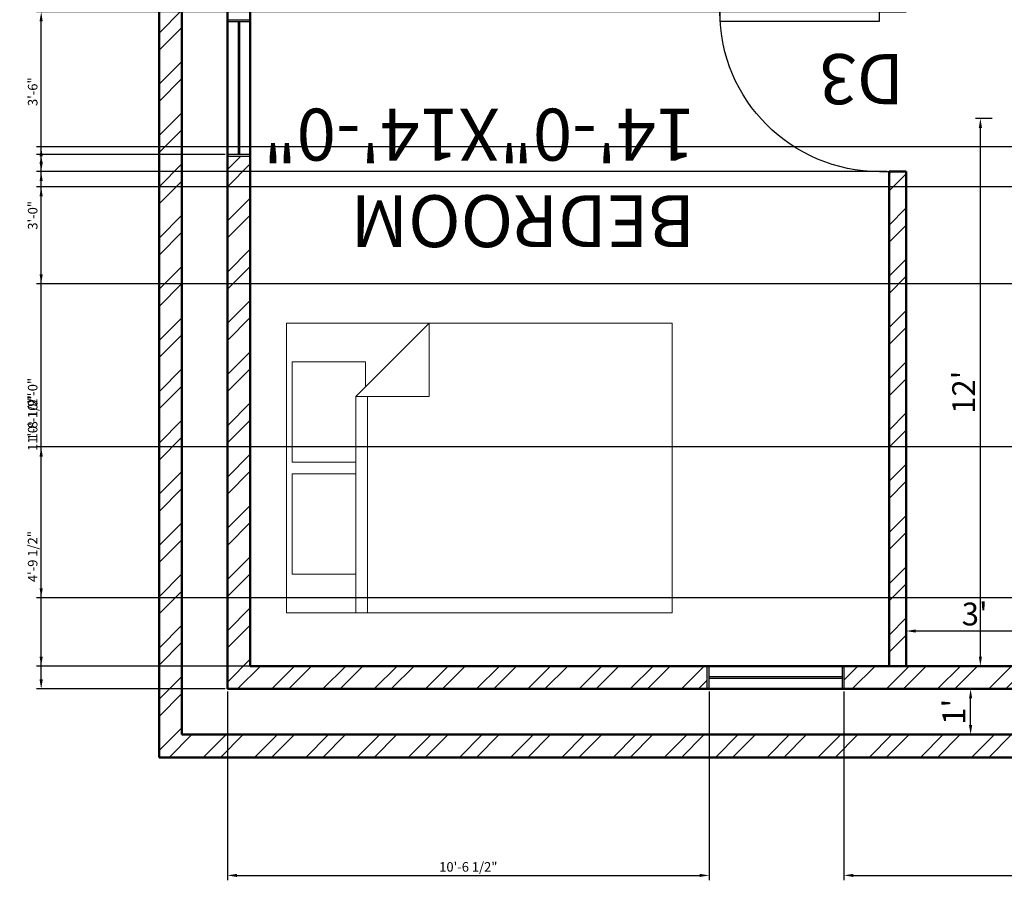
# Model space of a CAD drawing. Units: inches. Extents: x 244 to 2800, y 1060 to 1700.
# Tile 6 of 13: x 1476 to 1735, y 1060 to 1287. Entities that reach past the tile are written whole.
import ezdxf

# ---------------------------------------------------------------- set-up
doc = ezdxf.new("R2010")
doc.units = ezdxf.units.IN
for name, color, linetype, lineweight in [('A-ANNO-DIMS', 2, 'Continuous', 18), ('A-ANNO-TEXT', 1, 'Continuous', 18), ('A-DOOR', 5, 'Continuous', 25), ('A-FURN', 9, 'Continuous', 18), ('A-GLAZ', 3, 'Continuous', 25), ('A-WALL', 7, 'Continuous', 50), ('A-WALL-PATT', 8, 'Continuous', 13)]:
    doc.layers.add(name, color=color, linetype=linetype, lineweight=lineweight)
doc.styles.get("Standard").update_dxf_attribs({"font": 'arial.ttf'})
doc.dimstyles.new('ISO-25', dxfattribs={"dimtxt": 2.5, "dimasz": 2.5, "dimexe": 1.25, "dimexo": 0.625, "dimtad": 1, "dimlunit": 4, "dimtxsty": 'Standard', "dimcen": 2.5, "dimadec": 0, "dimazin": 0, "dimtfac": 1, "dimtmove": 0, "dimatfit": 3, "dimfxl": 1, "dimarcsym": 0})

# ---------------------------------------------------------------- blocks, each defined once
blk = doc.blocks.new('*U2')
for p, q in [((0, 0), (0, -5)), ((30, 0), (30, -5))]:
    blk.add_line(p, q)
blk.add_lwpolyline([(0, 0), (0, 30), (1.75, 30), (1.75, 0)], close=True)
blk.add_arc((0, 0), 30, 0, 90)
blk = doc.blocks.new('Bed - Queen')
for p, q in [((0, -80.00003), (0, 0)), ((0, 0), (59.99999, 0)), ((59.99999, 0), (59.99999, -80.00003)), ((7.99999, -1.2), (28.79998, -1.2)), ((7.99999, -14.4), (7.99999, -1.2)), ((28.79998, -1.2), (28.79998, -14.4)), ((31.19999, -1.2), (51.99999, -1.2)), ((31.19999, -14.4), (31.19999, -1.2)), ((51.99999, -1.2), (51.99999, -16.4)), ((0, -14.4), (44.8, -14.4)), ((59.99999, -29.6), (44.8, -14.4)), ((44.8, -14.4), (44.8, -29.6)), ((44.8, -16.8), (0, -16.8)), ((51.99999, -16.4), (46.79936, -16.4)), ((44.8, -29.6), (59.99999, -29.6)), ((59.99999, -80.00003), (0, -80.00003))]:
    blk.add_line(p, q)
blk = doc.blocks.new('*D37')
at = {"layer": 'A-ANNO-DIMS', "color": 0, "lineweight": -2, "transparency": 16777216}
for p, q in [((1731.11, 1110.99), (1724.58, 1110.99)), ((1725.83, 1101.49), (1725.83, 1108.49)), ((1731.11, 1098.99), (1724.58, 1098.99))]:
    blk.add_line(p, q, dxfattribs=at)
at = {"layer": 'A-ANNO-DIMS', "color": 0, "transparency": 16777216}
for points in [[(1725.42, 1108.49), (1726.25, 1108.49), (1725.83, 1110.99)], [(1725.42, 1101.49), (1726.25, 1101.49), (1725.83, 1098.99)]]:
    blk.add_solid(points, dxfattribs=at)
at = {"layer": 'Defpoints', "color": 0, "transparency": 16777216}
for p in [(1725.83, 1110.99), (1731.74, 1110.99), (1731.74, 1098.99)]:
    blk.add_point(p, dxfattribs=at)
at = {"layer": 'A-ANNO-DIMS', "color": 0, "transparency": 16777216, "insert": (1722.2, 1104.99), "char_height": 6, "attachment_point": 5, "rotation": 90}
blk.add_mtext("1'", dxfattribs=at)
blk = doc.blocks.new('*D38')
at = {"layer": 'A-ANNO-DIMS', "color": 0, "lineweight": -2, "transparency": 16777216}
for p, q in [((1708.9, 1124.22), (1708.9, 1127.48)), ((1744.9, 1124.22), (1744.9, 1127.48)), ((1742.4, 1126.23), (1711.4, 1126.23))]:
    blk.add_line(p, q, dxfattribs=at)
at = {"layer": 'A-ANNO-DIMS', "color": 0, "transparency": 16777216}
for points in [[(1711.4, 1126.65), (1711.4, 1125.81), (1708.9, 1126.23)], [(1742.4, 1126.65), (1742.4, 1125.81), (1744.9, 1126.23)]]:
    blk.add_solid(points, dxfattribs=at)
at = {"layer": 'Defpoints', "color": 0, "transparency": 16777216}
for p in [(1708.9, 1126.23), (1708.9, 1123.59), (1744.9, 1123.59)]:
    blk.add_point(p, dxfattribs=at)
at = {"layer": 'A-ANNO-DIMS', "color": 0, "transparency": 16777216, "insert": (1726.9, 1129.92), "char_height": 6, "attachment_point": 5}
blk.add_mtext("3'", dxfattribs=at)
blk = doc.blocks.new('*D39')
at = {"layer": 'A-ANNO-DIMS', "color": 0, "lineweight": -2, "transparency": 16777216}
for p, q in [((1731.52, 1260.99), (1727.15, 1260.99)), ((1728.4, 1119.49), (1728.4, 1258.49)), ((1731.92, 1116.99), (1727.15, 1116.99))]:
    blk.add_line(p, q, dxfattribs=at)
at = {"layer": 'A-ANNO-DIMS', "color": 0, "transparency": 16777216}
for points in [[(1727.99, 1258.49), (1728.82, 1258.49), (1728.4, 1260.99)], [(1727.99, 1119.49), (1728.82, 1119.49), (1728.4, 1116.99)]]:
    blk.add_solid(points, dxfattribs=at)
at = {"layer": 'Defpoints', "color": 0, "transparency": 16777216}
for p in [(1728.4, 1260.99), (1732.15, 1260.99), (1732.55, 1116.99)]:
    blk.add_point(p, dxfattribs=at)
at = {"layer": 'A-ANNO-DIMS', "color": 0, "transparency": 16777216, "insert": (1724.77, 1188.99), "char_height": 6, "attachment_point": 5, "rotation": 90}
blk.add_mtext("12'", dxfattribs=at)
blk = doc.blocks.new('WIN-36')
for p, q in [((0, 0), (0, 6)), ((0, 6), (35.94, 6)), ((35.94, 6), (35.94, 0)), ((35.94, 0), (0, 0))]:
    blk.add_line(p, q)
blk = doc.blocks.new('*D81')
at = {"layer": 'A-ANNO-DIMS', "color": 0, "lineweight": -2, "transparency": 16777216}
for p, q in [((1529.77, 1251.47), (1480.15, 1251.47)), ((1481.4, 1113.49), (1481.4, 1248.97)), ((1529.77, 1110.99), (1480.15, 1110.99))]:
    blk.add_line(p, q, dxfattribs=at)
at = {"layer": 'A-ANNO-DIMS', "color": 0, "transparency": 16777216}
for points in [[(1480.98, 1248.97), (1481.81, 1248.97), (1481.4, 1251.47)], [(1480.98, 1113.49), (1481.81, 1113.49), (1481.4, 1110.99)]]:
    blk.add_solid(points, dxfattribs=at)
at = {"layer": 'Defpoints', "color": 0, "transparency": 16777216}
for p in [(1481.4, 1251.47), (1530.4, 1251.47), (1530.4, 1110.99)]:
    blk.add_point(p, dxfattribs=at)
at = {"layer": 'A-ANNO-DIMS', "color": 0, "transparency": 16777216, "insert": (1479.48, 1181.23), "char_height": 2.5, "attachment_point": 5, "rotation": 90}
blk.add_mtext('11\'-8 1/2"', dxfattribs=at)
blk = doc.blocks.new('*D85')
at = {"layer": 'A-ANNO-DIMS', "color": 0, "lineweight": -2, "transparency": 16777216}
for p, q in [((1537.02, 1291.99), (2024.65, 1291.99)), ((2023.4, 1119.49), (2023.4, 1289.49)), ((1537.02, 1116.99), (2024.65, 1116.99))]:
    blk.add_line(p, q, dxfattribs=at)
at = {"layer": 'A-ANNO-DIMS', "color": 0, "transparency": 16777216}
for points in [[(2022.98, 1289.49), (2023.81, 1289.49), (2023.4, 1291.99)], [(2022.98, 1119.49), (2023.81, 1119.49), (2023.4, 1116.99)]]:
    blk.add_solid(points, dxfattribs=at)
at = {"layer": 'Defpoints', "color": 0, "transparency": 16777216}
for p in [(1536.4, 1291.99), (2023.4, 1291.99), (1536.4, 1116.99)]:
    blk.add_point(p, dxfattribs=at)
at = {"layer": 'A-ANNO-DIMS', "color": 0, "transparency": 16777216, "insert": (2021.52, 1204.49), "char_height": 2.5, "attachment_point": 5, "rotation": 90}
blk.add_mtext('14\'-7"', dxfattribs=at)
blk = doc.blocks.new('*D91')
at = {"layer": 'A-ANNO-DIMS', "color": 0, "lineweight": -2, "transparency": 16777216}
for p, q in [((1703.77, 1246.99), (1480.15, 1246.99)), ((1481.4, 1119.49), (1481.4, 1244.49)), ((1703.77, 1116.99), (1480.15, 1116.99))]:
    blk.add_line(p, q, dxfattribs=at)
at = {"layer": 'A-ANNO-DIMS', "color": 0, "transparency": 16777216}
for points in [[(1480.98, 1244.49), (1481.81, 1244.49), (1481.4, 1246.99)], [(1480.98, 1119.49), (1481.81, 1119.49), (1481.4, 1116.99)]]:
    blk.add_solid(points, dxfattribs=at)
at = {"layer": 'Defpoints', "color": 0, "transparency": 16777216}
for p in [(1481.4, 1246.99), (1704.4, 1246.99), (1704.4, 1116.99)]:
    blk.add_point(p, dxfattribs=at)
at = {"layer": 'A-ANNO-DIMS', "color": 0, "transparency": 16777216, "insert": (1479.49, 1181.99), "char_height": 2.5, "attachment_point": 5, "rotation": 90}
blk.add_mtext('10\'-10"', dxfattribs=at)
blk = doc.blocks.new('*D92')
at = {"layer": 'A-ANNO-DIMS', "color": 0, "lineweight": -2, "transparency": 16777216}
for p, q in [((1703.77, 1288.99), (1480.15, 1288.99)), ((1481.4, 1249.49), (1481.4, 1286.49)), ((1703.77, 1246.99), (1480.15, 1246.99))]:
    blk.add_line(p, q, dxfattribs=at)
at = {"layer": 'A-ANNO-DIMS', "color": 0, "transparency": 16777216}
for points in [[(1480.98, 1286.49), (1481.81, 1286.49), (1481.4, 1288.99)], [(1480.98, 1249.49), (1481.81, 1249.49), (1481.4, 1246.99)]]:
    blk.add_solid(points, dxfattribs=at)
at = {"layer": 'Defpoints', "color": 0, "transparency": 16777216}
for p in [(1481.4, 1288.99), (1704.4, 1288.99), (1704.4, 1246.99)]:
    blk.add_point(p, dxfattribs=at)
at = {"layer": 'A-ANNO-DIMS', "color": 0, "transparency": 16777216, "insert": (1479.49, 1267.99), "char_height": 2.5, "attachment_point": 5, "rotation": 90}
blk.add_mtext('3\'-6"', dxfattribs=at)
blk = doc.blocks.new('*D94')
at = {"layer": 'A-ANNO-DIMS', "color": 0, "lineweight": -2, "transparency": 16777216}
for p, q in [((1530.4, 1110.36), (1530.4, 1060.74)), ((1657.07, 1110.36), (1657.07, 1060.74)), ((1532.9, 1061.99), (1654.57, 1061.99))]:
    blk.add_line(p, q, dxfattribs=at)
at = {"layer": 'A-ANNO-DIMS', "color": 0, "transparency": 16777216}
for points in [[(1532.9, 1062.4), (1532.9, 1061.57), (1530.4, 1061.99)], [(1654.57, 1062.4), (1654.57, 1061.57), (1657.07, 1061.99)]]:
    blk.add_solid(points, dxfattribs=at)
at = {"layer": 'Defpoints', "color": 0, "transparency": 16777216}
for p in [(1530.4, 1110.99), (1657.07, 1110.99), (1657.07, 1061.99)]:
    blk.add_point(p, dxfattribs=at)
at = {"layer": 'A-ANNO-DIMS', "color": 0, "transparency": 16777216, "insert": (1593.74, 1063.9), "char_height": 2.5, "attachment_point": 5}
blk.add_mtext('10\'-6 1/2"', dxfattribs=at)
blk = doc.blocks.new('*D95')
at = {"layer": 'A-ANNO-DIMS', "color": 0, "lineweight": -2, "transparency": 16777216}
for p, q in [((1692.52, 1110.36), (1692.52, 1060.74)), ((1795.9, 1110.36), (1795.9, 1060.74)), ((1695.02, 1061.99), (1793.4, 1061.99))]:
    blk.add_line(p, q, dxfattribs=at)
at = {"layer": 'A-ANNO-DIMS', "color": 0, "transparency": 16777216}
for points in [[(1695.02, 1062.4), (1695.02, 1061.57), (1692.52, 1061.99)], [(1793.4, 1062.4), (1793.4, 1061.57), (1795.9, 1061.99)]]:
    blk.add_solid(points, dxfattribs=at)
at = {"layer": 'Defpoints', "color": 0, "transparency": 16777216}
for p in [(1692.52, 1110.99), (1795.9, 1110.99), (1795.9, 1061.99)]:
    blk.add_point(p, dxfattribs=at)
at = {"layer": 'A-ANNO-DIMS', "color": 0, "transparency": 16777216, "insert": (1744.21, 1063.9), "char_height": 2.5, "attachment_point": 5}
blk.add_mtext('8\'-7 1/2"', dxfattribs=at)
blk = doc.blocks.new('*D103')
at = {"layer": 'A-ANNO-DIMS', "color": 0, "lineweight": -2, "transparency": 16777216}
for p, q in [((1985.77, 1242.99), (1480.15, 1242.99)), ((1481.4, 1137.49), (1481.4, 1240.49)), ((1985.77, 1134.99), (1480.15, 1134.99))]:
    blk.add_line(p, q, dxfattribs=at)
at = {"layer": 'A-ANNO-DIMS', "color": 0, "transparency": 16777216}
for points in [[(1480.98, 1240.49), (1481.81, 1240.49), (1481.4, 1242.99)], [(1480.98, 1137.49), (1481.81, 1137.49), (1481.4, 1134.99)]]:
    blk.add_solid(points, dxfattribs=at)
at = {"layer": 'Defpoints', "color": 0, "transparency": 16777216}
for p in [(1481.4, 1242.99), (1986.4, 1242.99), (1986.4, 1134.99)]:
    blk.add_point(p, dxfattribs=at)
at = {"layer": 'A-ANNO-DIMS', "color": 0, "transparency": 16777216, "insert": (1479.49, 1188.99), "char_height": 2.5, "attachment_point": 5, "rotation": 90}
blk.add_mtext('9\'-0"', dxfattribs=at)
blk = doc.blocks.new('*D105')
at = {"layer": 'A-ANNO-DIMS', "color": 0, "lineweight": -2, "transparency": 16777216}
for p, q in [((1831.27, 1253.49), (1480.15, 1253.49)), ((1481.4, 1219.99), (1481.4, 1250.99)), ((1831.27, 1217.49), (1480.15, 1217.49))]:
    blk.add_line(p, q, dxfattribs=at)
at = {"layer": 'A-ANNO-DIMS', "color": 0, "transparency": 16777216}
for points in [[(1480.98, 1250.99), (1481.81, 1250.99), (1481.4, 1253.49)], [(1480.98, 1219.99), (1481.81, 1219.99), (1481.4, 1217.49)]]:
    blk.add_solid(points, dxfattribs=at)
at = {"layer": 'Defpoints', "color": 0, "transparency": 16777216}
for p in [(1481.4, 1253.49), (1831.9, 1253.49), (1831.9, 1217.49)]:
    blk.add_point(p, dxfattribs=at)
at = {"layer": 'A-ANNO-DIMS', "color": 0, "transparency": 16777216, "insert": (1479.49, 1235.49), "char_height": 2.5, "attachment_point": 5, "rotation": 90}
blk.add_mtext('3\'-0"', dxfattribs=at)
blk = doc.blocks.new('*D106')
at = {"layer": 'A-ANNO-DIMS', "color": 0, "lineweight": -2, "transparency": 16777216}
for p, q in [((1895.77, 1174.6), (1480.15, 1174.6)), ((1481.4, 1119.49), (1481.4, 1172.1)), ((1895.77, 1116.99), (1480.15, 1116.99))]:
    blk.add_line(p, q, dxfattribs=at)
at = {"layer": 'A-ANNO-DIMS', "color": 0, "transparency": 16777216}
for points in [[(1480.98, 1172.1), (1481.81, 1172.1), (1481.4, 1174.6)], [(1480.98, 1119.49), (1481.81, 1119.49), (1481.4, 1116.99)]]:
    blk.add_solid(points, dxfattribs=at)
at = {"layer": 'Defpoints', "color": 0, "transparency": 16777216}
for p in [(1481.4, 1174.6), (1896.4, 1174.6), (1896.4, 1116.99)]:
    blk.add_point(p, dxfattribs=at)
at = {"layer": 'A-ANNO-DIMS', "color": 0, "transparency": 16777216, "insert": (1479.48, 1145.79), "char_height": 2.5, "attachment_point": 5, "rotation": 90}
blk.add_mtext('4\'-9 1/2"', dxfattribs=at)

msp = doc.modelspace()

# ---------------------------------------------------------------- hatches: boundary and pattern name
at = {"layer": 'A-WALL-PATT'}
h = msp.add_hatch(dxfattribs=at)
h.set_pattern_fill('ANSI32', color=256)
h.paths.add_polyline_path([(1992.396, 1092.986), (1992.396, 1632.986), (1512.396, 1632.986), (1512.396, 1092.986)])
h.paths.add_polyline_path([(1518.396, 1098.986), (1518.396, 1626.986), (1986.396, 1626.986), (1986.396, 1098.986), (1902.396, 1098.986)], flags=16)
h.paths.add_polyline_path([(1795.896, 1110.986), (1530.396, 1110.986), (1530.396, 1551.986), (1521.7, 1551.986), (1521.7, 1623.986), (1605.7, 1623.986), (1605.7, 1551.986), (1781.396, 1551.986), (1781.396, 1545.986), (1708.896, 1545.986), (1708.896, 1532.64), (1704.396, 1532.64), (1704.396, 1545.986), (1536.396, 1545.986), (1536.396, 1372.986), (1671.396, 1372.986), (1671.396, 1368.486), (1621.896, 1368.486), (1621.896, 1296.486), (1704.396, 1296.486), (1704.396, 1368.486), (1701.396, 1368.486), (1701.396, 1372.986), (1704.396, 1372.986), (1704.396, 1490.64), (1708.896, 1490.64), (1708.896, 1288.986), (1704.396, 1288.986), (1704.396, 1291.986), (1569.396, 1291.986), (1569.396, 1296.486), (1618.896, 1296.486), (1618.896, 1368.486), (1536.396, 1368.486), (1536.396, 1296.486), (1539.396, 1296.486), (1539.396, 1291.986), (1536.396, 1291.986), (1536.396, 1116.986), (1704.396, 1116.986), (1704.396, 1246.986), (1708.896, 1246.986), (1708.896, 1116.986), (1744.896, 1116.986), (1744.896, 1260.986), (1780.896, 1260.986), (1785.396, 1260.986), (1785.396, 1205.486), (1831.896, 1205.486), (1831.896, 1217.486), (1836.396, 1217.486), (1836.396, 1205.486), (1896.396, 1205.486), (1896.396, 1265.486), (1836.396, 1265.486), (1836.396, 1253.486), (1831.896, 1253.486), (1831.896, 1269.986), (1896.396, 1269.986), (1896.396, 1472.64), (1902.396, 1472.64), (1902.396, 1242.986), (1938.396, 1242.986), (1938.396, 1134.986), (1950.396, 1134.986), (1950.396, 1242.986), (1986.396, 1242.986), (1986.396, 1134.986), (1902.396, 1134.986), (1902.396, 1110.986), (1831.896, 1110.986), (1831.896, 1116.986), (1896.396, 1116.986), (1896.396, 1200.986), (1785.396, 1200.986), (1785.396, 1116.986), (1795.896, 1116.986)], flags=0)
h.paths.add_polyline_path([(1780.896, 1116.986), (1744.896, 1116.986), (1744.896, 1260.986), (1780.896, 1260.986)], flags=0)
h.paths.add_polyline_path([(1863.351, 1110.986), (1863.351, 1116.986), (1887.296, 1116.986), (1887.296, 1110.986)], flags=0)
h.paths.add_polyline_path([(1863.851, 1114.186), (1886.796, 1114.186), (1886.796, 1113.786), (1863.851, 1113.786)], flags=0)
h.paths.add_polyline_path([(1896.396, 1174.102), (1896.396, 1198.047), (1902.396, 1198.047), (1902.396, 1174.102)], flags=0)
h.paths.add_polyline_path([(1902.396, 1174.602), (1899.196, 1174.602), (1899.196, 1197.547), (1902.396, 1197.547)], flags=0)
h.paths.add_polyline_path([(1692.519, 1110.986), (1656.574, 1110.986), (1656.574, 1116.986), (1692.519, 1116.986)], flags=0)
h.paths.add_polyline_path([(1819.776, 1376.187), (1819.776, 1410.382, -0.249194), (1838.546, 1410.382), (1838.546, 1376.187, -0.249194)], flags=0)
h.paths.add_polyline_path([(1536.396, 1250.972), (1530.396, 1250.972), (1530.396, 1286.917), (1536.396, 1286.917)], flags=0)
h.paths.add_polyline_path([(1896.396, 1405.581), (1896.396, 1453.526), (1902.396, 1453.526), (1902.396, 1405.581)], flags=0)
h.paths.add_polyline_path([(1536.396, 1322.935), (1530.396, 1322.935), (1530.396, 1346.88), (1536.396, 1346.88)], flags=0)
h.paths.add_polyline_path([(1533.196, 1323.435), (1533.196, 1346.38), (1533.596, 1346.38), (1533.596, 1323.435)], flags=0)
h.paths.add_polyline_path([(1896.396, 1545.986), (1841.396, 1545.986), (1841.396, 1551.986), (1902.396, 1551.986), (1902.396, 1532.64), (1896.396, 1532.64)], flags=0)
h.paths.add_polyline_path([(1756.808, 1545.986), (1732.863, 1545.986), (1732.863, 1551.986), (1756.808, 1551.986)], flags=0)
h.paths.add_polyline_path([(1756.308, 1548.786), (1733.363, 1548.786), (1733.363, 1551.986), (1756.308, 1551.986)], flags=0)
h.paths.add_polyline_path([(1673.743, 1545.986), (1637.798, 1545.986), (1637.798, 1551.986), (1673.743, 1551.986)], flags=0)
h.paths.add_polyline_path([(1536.396, 1503.969), (1530.396, 1503.969), (1530.396, 1539.914), (1536.396, 1539.914)], flags=0)
h.paths.add_polyline_path([(1896.341, 1192.868), (1881.737, 1192.868), (1881.737, 1181.273), (1896.341, 1181.273)], flags=8)
h.paths.add_polyline_path([(1882.893, 1112.542), (1868.29, 1112.542), (1868.29, 1100.947), (1882.893, 1100.947)], flags=8)
h.paths.add_polyline_path([(1531.898, 1340.208), (1517.295, 1340.208), (1517.295, 1328.613), (1531.898, 1328.613)], flags=24)
h.paths.add_polyline_path([(1662.207, 1564.332), (1647.603, 1564.332), (1647.603, 1552.737), (1662.207, 1552.737)], flags=8)
h.paths.add_polyline_path([(1750.605, 1565.018), (1736.001, 1565.018), (1736.001, 1553.424), (1750.605, 1553.424)], flags=8)
h.paths.add_polyline_path([(1919.351, 1440.326), (1904.748, 1440.326), (1904.748, 1428.731), (1919.351, 1428.731)], flags=8)
h.paths.add_polyline_path([(1827.662, 1149.994), (1797.512, 1149.994), (1797.512, 1122.813), (1827.662, 1122.813)], flags=8)
h.paths.add_polyline_path([(1826.683, 1247.85), (1796.533, 1247.85), (1796.533, 1220.668), (1826.683, 1220.668)], flags=8)
h.paths.add_polyline_path([(1713.043, 1285.137), (1682.893, 1285.137), (1682.893, 1257.956), (1713.043, 1257.956)], flags=8)
h.paths.add_polyline_path([(1567.301, 1310.129), (1537.151, 1310.129), (1537.151, 1282.948), (1567.301, 1282.948)], flags=8)
h.paths.add_polyline_path([(1699.655, 1386.046), (1669.505, 1386.046), (1669.505, 1358.865), (1699.655, 1358.865)], flags=8)
h.paths.add_polyline_path([(1716.254, 1527.375), (1686.103, 1527.375), (1686.103, 1500.194), (1716.254, 1500.194)], flags=8)
h.paths.add_polyline_path([(1822.088, 1577.207), (1791.938, 1577.207), (1791.938, 1550.026), (1822.088, 1550.026)], flags=8)
h.paths.add_polyline_path([(1931.716, 1518.23), (1901.565, 1518.23), (1901.565, 1491.049), (1931.716, 1491.049)], flags=8)
h.paths.add_polyline_path([(1636.272, 1573.477), (1636.272, 1615.869), (1613.819, 1615.869), (1613.819, 1573.477)], flags=8)
h.paths.add_polyline_path([(1968.141, 1266.003), (1911.144, 1266.003), (1911.144, 1252.05), (1968.141, 1252.05)], flags=8)
h.paths.add_polyline_path([(1783.26, 1275.202), (1745.711, 1275.202), (1745.711, 1261.249), (1783.26, 1261.249)], flags=8)
h.paths.add_polyline_path([(1753.522, 1456.095), (1753.522, 1338.024), (1798.876, 1338.024), (1798.876, 1456.095)], flags=8)
h.paths.add_polyline_path([(1884.04, 1192.467), (1803.345, 1192.467), (1803.345, 1149.693), (1884.04, 1149.693)], flags=8)
h.paths.add_polyline_path([(1863.426, 1264.753), (1863.426, 1209.557), (1892.661, 1209.557), (1892.661, 1264.753)], flags=8)
h.paths.add_polyline_path([(1594.411, 1361.178), (1536.688, 1361.178), (1536.688, 1330.387), (1594.411, 1330.387)], flags=8)
h.paths.add_polyline_path([(1695.984, 1342.402), (1638.262, 1342.402), (1638.262, 1311.611), (1695.984, 1311.611)], flags=8)
h.paths.add_polyline_path([(1654.435, 1540.65), (1537.752, 1540.65), (1537.752, 1489.721), (1654.435, 1489.721)], flags=8)
h.paths.add_polyline_path([(1658.864, 1271.272), (1542.182, 1271.272), (1542.182, 1220.343), (1658.864, 1220.343)], flags=8)
h = msp.add_hatch(dxfattribs=at)
h.set_pattern_fill('ANSI32', color=256)
h.paths.add_polyline_path([(1656.574, 1116.986), (1536.396, 1116.986), (1536.396, 1250.972), (1530.396, 1250.972), (1530.396, 1110.986), (1656.574, 1110.986)])
h = msp.add_hatch(dxfattribs=at)
h.set_pattern_fill('ANSI32', color=256)
h.paths.add_polyline_path([(1708.896, 1246.986), (1704.396, 1246.986), (1704.396, 1116.986), (1708.896, 1116.986)])
h = msp.add_hatch(dxfattribs=at)
h.set_pattern_fill('ANSI32', color=256)
h.paths.add_polyline_path([(1795.896, 1116.986), (1692.519, 1116.986), (1692.519, 1110.986), (1795.896, 1110.986), (1795.896, 1113.986)])

# ---------------------------------------------------------------- linework, layer by layer
at = {"layer": 'A-GLAZ'}
for p, q in [((1530.396, 1286.417), (1536.396, 1286.417)), ((1533.196, 1286.417), (1533.196, 1251.472)), ((1533.596, 1286.417), (1533.596, 1251.472)), ((1536.396, 1251.472), (1530.396, 1251.472)), ((1657.074, 1110.986), (1657.074, 1116.986)), ((1692.019, 1116.986), (1692.019, 1110.986)), ((1692.019, 1114.186), (1657.074, 1114.186)), ((1692.019, 1113.786), (1657.074, 1113.786))]:
    msp.add_line(p, q, dxfattribs=at)
at = {"layer": 'A-WALL'}
for p, q in [((1512.396, 1632.986), (1512.396, 1092.986)), ((1518.396, 1626.986), (1518.396, 1098.986)), ((1530.396, 1551.986), (1530.396, 1110.986)), ((1536.396, 1291.986), (1536.396, 1116.986)), ((1708.896, 1246.986), (1704.396, 1246.986)), ((1704.396, 1246.986), (1704.396, 1116.986)), ((1708.896, 1246.986), (1708.896, 1116.986)), ((1536.396, 1116.986), (1795.896, 1116.986)), ((1530.396, 1110.986), (1795.896, 1110.986)), ((1518.396, 1098.986), (1986.396, 1098.986)), ((1512.396, 1092.986), (1992.396, 1092.986))]:
    msp.add_line(p, q, dxfattribs=at)

# ---------------------------------------------------------------- block references
at = {"layer": 'A-DOOR', "xscale": -1.399999999999999, "yscale": 1.399999999999999, "zscale": 1.399999999999999, "rotation": 90}
msp.add_blockref('*U2', (1701.896, 1288.986), dxfattribs=at)
at = {"layer": 'A-FURN', "xscale": 1.268227082860182, "yscale": 1.268227082860182, "zscale": 1.268227082860182, "rotation": 90}
msp.add_blockref('Bed - Queen', (1545.908, 1131.036), dxfattribs=at)
at = {"layer": 'A-GLAZ'}
for p, rotation in [((1530.396, 1286.917), 269.9999999999986), ((1692.519, 1116.986), 180)]:
    msp.add_blockref('WIN-36', p, dxfattribs=dict(at, rotation=rotation))

# ---------------------------------------------------------------- texts
at = {"layer": 'A-ANNO-TEXT', "attachment_point": 1, "rotation": 180}
for s, width, gutter_width, insert, char_height in [('D3', 20.58737, 65.951, (1708.324, 1264.69), 13.1902), ('BEDROOM\\P14\'-0"X14\'-0"', 25.27039, 68.243, (1653.376, 1227.126), 13.64851)]:
    msp.add_mtext_dynamic_manual_height_columns(s, width=width, gutter_width=gutter_width, heights=[0], dxfattribs=dict(at, insert=insert, char_height=char_height))

# ---------------------------------------------------------------- dimensions: what is measured, and where the dimension line sits
at = {"layer": 'A-ANNO-DIMS'}
for base, p1, p2, override, picture, middle in [((2023.396, 1291.986), (1536.396, 1116.986), (1536.396, 1291.986), {"dimdec": 1, "dimlfac": 1, "dimrnd": 0, "dimzin": 1, "dimdsep": 46, "dimlunit": 4, "dimfrac": 2}, '*D85', (2021.516, 1204.486)), ((1481.396, 1288.986), (1704.396, 1246.986), (1704.396, 1288.986), {"dimdec": 1, "dimlfac": 1, "dimrnd": 0, "dimzin": 1, "dimdsep": 46, "dimlunit": 4, "dimfrac": 2}, '*D92', (1479.493, 1267.986)), ((1728.404, 1260.986), (1732.547, 1116.986), (1732.149, 1260.986), {"dimtxt": 6, "dimclrd": 0, "dimclre": 0, "dimclrt": 0}, '*D39', (1724.767, 1188.986)), ((1481.396, 1253.486), (1831.896, 1217.486), (1831.896, 1253.486), {"dimdec": 1, "dimlfac": 1, "dimrnd": 0, "dimzin": 1, "dimdsep": 46, "dimlunit": 4, "dimfrac": 2}, '*D105', (1479.493, 1235.486)), ((1481.396, 1251.472), (1530.396, 1110.986), (1530.396, 1251.472), {"dimdec": 1, "dimlfac": 1, "dimrnd": 0, "dimzin": 1, "dimdsep": 46, "dimlunit": 4, "dimfrac": 2}, '*D81', (1479.478, 1181.229)), ((1481.396, 1246.986), (1704.396, 1116.986), (1704.396, 1246.986), {"dimdec": 1, "dimlfac": 1, "dimrnd": 0, "dimzin": 1, "dimdsep": 46, "dimlunit": 4, "dimfrac": 2}, '*D91', (1479.494, 1181.986)), ((1481.396, 1242.986), (1986.396, 1134.986), (1986.396, 1242.986), {"dimdec": 1, "dimlfac": 1, "dimrnd": 0, "dimzin": 1, "dimdsep": 46, "dimlunit": 4, "dimfrac": 2}, '*D103', (1479.494, 1188.986)), ((1481.396, 1174.602), (1896.396, 1116.986), (1896.396, 1174.602), {"dimdec": 1, "dimlfac": 1, "dimrnd": 0, "dimzin": 1, "dimdsep": 46, "dimlunit": 4, "dimfrac": 2}, '*D106', (1479.478, 1145.794)), ((1725.835, 1110.986), (1731.738, 1098.986), (1731.738, 1110.986), {"dimtxt": 6, "dimclrd": 0, "dimclre": 0, "dimclrt": 0}, '*D37', (1722.198, 1104.986))]:
    dim = msp.add_linear_dim(base=base, p1=p1, p2=p2, angle=90, dimstyle='ISO-25', override=override, dxfattribs=at)
    dim.commit()
    dim.dimension.update_dxf_attribs({"geometry": picture, "text_midpoint": middle})
for base, p1, p2, override, picture, middle in [((1708.896, 1126.23), (1744.896, 1123.591), (1708.896, 1123.591), {"dimtxt": 6, "dimclrd": 0, "dimclre": 0, "dimclrt": 0}, '*D38', (1726.896, 1129.921)), ((1657.074, 1061.986), (1530.396, 1110.986), (1657.074, 1110.986), {"dimdec": 1, "dimlfac": 1, "dimrnd": 0, "dimzin": 1, "dimdsep": 46, "dimlunit": 4, "dimfrac": 2}, '*D94', (1593.735, 1063.904)), ((1795.896, 1061.986), (1692.519, 1110.986), (1795.896, 1110.986), {"dimdec": 1, "dimlfac": 1, "dimrnd": 0, "dimzin": 1, "dimdsep": 46, "dimlunit": 4, "dimfrac": 2}, '*D95', (1744.208, 1063.904))]:
    dim = msp.add_linear_dim(base=base, p1=p1, p2=p2, dimstyle='ISO-25', override=override, dxfattribs=at)
    dim.commit()
    dim.dimension.update_dxf_attribs({"geometry": picture, "text_midpoint": middle})

doc.saveas('drawing.dxf')
